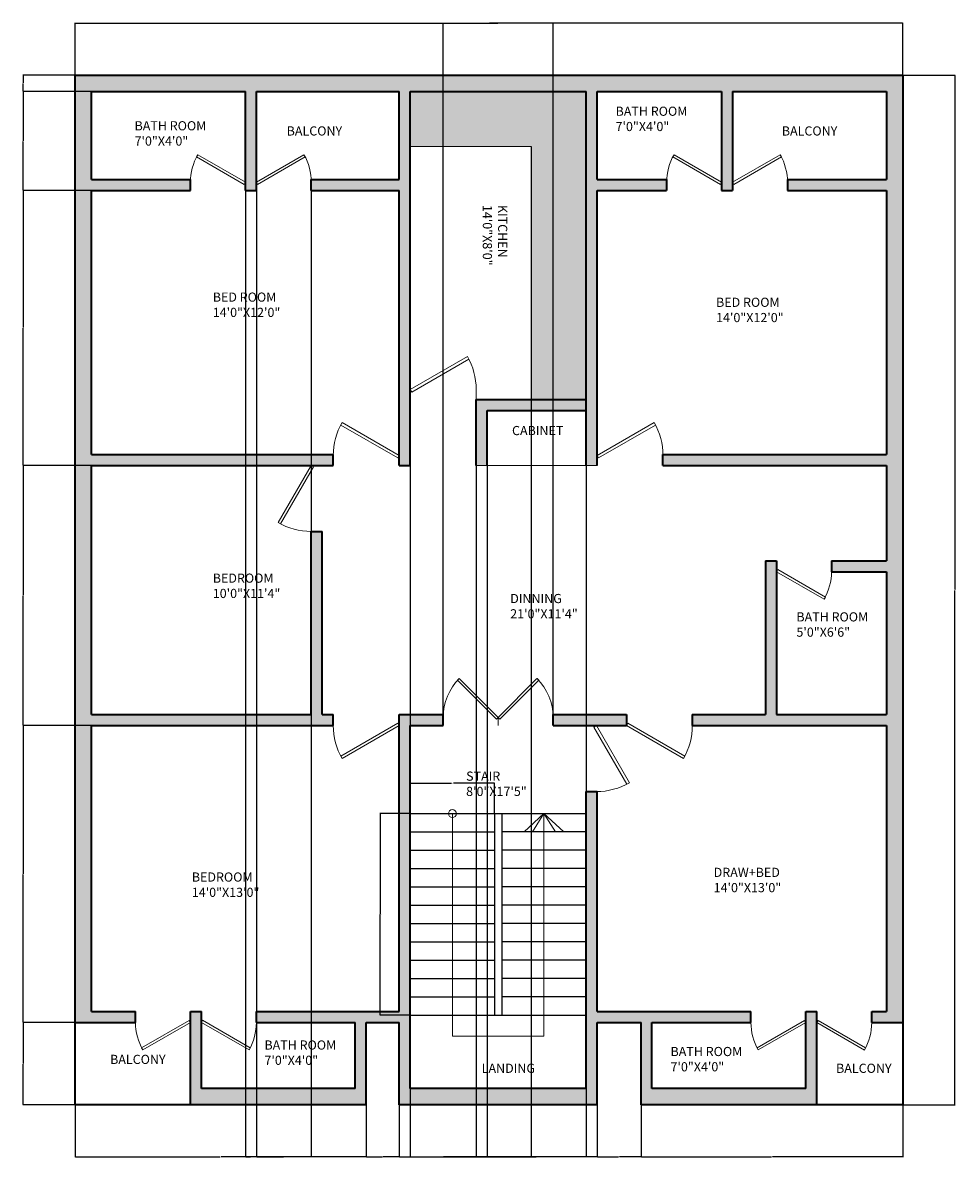
# Model space of a CAD drawing. Units: feet. Extents: x 3441 to 3951, y 1231 to 1850.
import ezdxf

# ---------------------------------------------------------------- set-up
doc = ezdxf.new("R2010")
doc.units = ezdxf.units.FT
for name, color, linetype, lineweight in [('A-ANNO-DIMS', 2, 'Continuous', 18), ('A-ANNO-SYMB', 130, 'Continuous', 13), ('A-AREA-IDEN', 170, 'Continuous', 18), ('A-FLOR-CASE', 7, 'Continuous', 18), ('A-FLOR-CASE-PATT', 8, 'Continuous', 13), ('A-WALL', 7, 'Continuous', 35), ('DOOR', 119, 'Continuous', 18), ('STAIR CASE', 130, 'Continuous', 25)]:
    doc.layers.add(name, color=color, linetype=linetype, lineweight=lineweight)
doc.layers.add('A-WALL-PATT', color=244, linetype='Continuous', lineweight=13, true_color=0x991b1e)
doc.styles.get("Standard").update_dxf_attribs({"font": 'arial.ttf'})
doc.dimstyles.get("Standard").update_dxf_attribs({"dimtxt": 0.18, "dimasz": 0.18, "dimexe": 0.18, "dimexo": 0.0625, "dimgap": 0.09, "dimtad": 0, "dimtih": 1, "dimtoh": 1, "dimdec": 4, "dimzin": 0, "dimdsep": 46, "dimtxsty": 'Standard', "dimcen": 0.09, "dimadec": 0, "dimazin": 0, "dimtfac": 1, "dimtdec": 4, "dimtofl": 0, "dimtmove": 0, "dimatfit": 3, "dimfxl": 1, "dimtolj": 1, "dimtzin": 0, "dimarcsym": 0})

# ---------------------------------------------------------------- blocks, each defined once
blk = doc.blocks.new('*U5')
for p, q in [((0, 0), (0, -6)), ((40, 0), (40, -6))]:
    blk.add_line(p, q)
blk.add_lwpolyline([(0, 0), (34.64, 20), (35.52, 18.48), (0.87, -1.52)], close=True)
blk.add_arc((0, 0), 40, 0, 30)
blk = doc.blocks.new('*U6')
for p, q in [((0, 0), (0, -6)), ((-40, 0), (-40, -6))]:
    blk.add_line(p, q)
blk.add_lwpolyline([(0, 0), (-34.64, 20), (-35.52, 18.48), (-0.88, -1.52)], close=True)
blk.add_arc((0, 0), 40, 150, 180)
blk = doc.blocks.new('*U4')
for p, q in [((0, 0), (0, -6)), ((-40, 0), (-40, -6))]:
    blk.add_line(p, q)
blk.add_lwpolyline([(0, 0), (-34.64, 20), (-35.52, 18.48), (-0.88, -1.52)], close=True)
blk.add_arc((0, 0), 40, 150, 180)
blk = doc.blocks.new('*U3')
for p, q in [((-40, 0), (-40, 6)), ((0, 0), (0, 6))]:
    blk.add_line(p, q)
blk.add_lwpolyline([(0, 0), (-34.64, -20), (-35.52, -18.48), (-0.87, 1.52)], close=True)
blk.add_arc((0, 0), 40, 180, 210)
blk = doc.blocks.new('*U2')
for p, q in [((0, 0), (0, 6)), ((40, 0), (40, 6))]:
    blk.add_line(p, q)
blk.add_lwpolyline([(0, 0), (34.64, -20), (35.52, -18.48), (0.87, 1.52)], close=True)
blk.add_arc((0, 0), 40, 330, 0)
blk = doc.blocks.new('*U7')
for p, q in [((0, 0), (0, 6)), ((40, 0), (40, 6))]:
    blk.add_line(p, q)
blk.add_lwpolyline([(0, 0), (34.64, -20), (35.52, -18.48), (0.87, 1.52)], close=True)
blk.add_arc((0, 0), 40, 330, 0)
blk = doc.blocks.new('*U9')
for p, q in [((-40, 0), (-40, 6)), ((0, 0), (0, 6))]:
    blk.add_line(p, q)
blk.add_lwpolyline([(0, 0), (-34.64, -20), (-35.52, -18.48), (-0.88, 1.52)], close=True)
blk.add_arc((0, 0), 40, 180, 210)
blk = doc.blocks.new('*U8')
for p, q in [((0, 0), (0, -6)), ((-40, 0), (-40, -6))]:
    blk.add_line(p, q)
blk.add_lwpolyline([(0, 0), (-34.64, 20), (-35.52, 18.48), (-0.88, -1.52)], close=True)
blk.add_arc((0, 0), 40, 150, 180)
blk = doc.blocks.new('*U10')
for p, q in [((0, 0), (0, -6)), ((40, 0), (40, -6))]:
    blk.add_line(p, q)
blk.add_lwpolyline([(0, 0), (28.28, 28.28), (29.52, 27.05), (1.24, -1.24)], close=True)
blk.add_arc((0, 0), 40, 0, 45)
blk = doc.blocks.new('STAIR-FLIGHT-46IN')
for p, q in [((46, 110), (46, 0)), ((0, 100), (46, 100)), ((0, 90), (46, 90)), ((0, 80), (46, 80)), ((0, 70), (46, 70)), ((0, 60), (46, 60)), ((0, 50), (46, 50)), ((0, 40), (46, 40)), ((0, 30), (46, 30)), ((0, 20), (46, 20)), ((0, 20), (46, 20)), ((0, 10), (46, 10))]:
    blk.add_line(p, q)
blk = doc.blocks.new('*D12')
at = {"layer": 'A-ANNO-DIMS', "color": 0, "lineweight": -2, "transparency": 16777216}
for p, q in [((3652.89, 1418.79), (3636.27, 1418.79)), ((3636.45, 1418.61), (3636.45, 1363.97)), ((3636.45, 1308.97), (3636.45, 1363.6)), ((3652.89, 1308.79), (3636.27, 1308.79))]:
    blk.add_line(p, q, dxfattribs=at)
at = {"layer": 'A-ANNO-DIMS', "color": 0, "transparency": 16777216}
for points in [[(3636.42, 1418.61), (3636.48, 1418.61), (3636.45, 1418.79)], [(3636.42, 1308.97), (3636.48, 1308.97), (3636.45, 1308.79)]]:
    blk.add_solid(points, dxfattribs=at)
at = {"layer": 'Defpoints', "color": 0, "transparency": 16777216}
for p in [(3636.45, 1418.79), (3652.95, 1418.79), (3652.95, 1308.79)]:
    blk.add_point(p, dxfattribs=at)
at = {"layer": 'A-ANNO-DIMS', "color": 0, "transparency": 16777216, "insert": (3636.45, 1363.79), "char_height": 0.18, "attachment_point": 5}
blk.add_mtext('\\A1;FLIGHT 110 TYP.', dxfattribs=at)
blk = doc.blocks.new('*D13')
at = {"layer": 'A-ANNO-DIMS', "color": 0, "lineweight": -2, "transparency": 16777216}
for p, q in [((3652.95, 1418.85), (3652.95, 1435.47)), ((3653.13, 1435.29), (3675.42, 1435.29)), ((3698.77, 1435.29), (3676.49, 1435.29)), ((3698.95, 1418.85), (3698.95, 1435.47))]:
    blk.add_line(p, q, dxfattribs=at)
at = {"layer": 'A-ANNO-DIMS', "color": 0, "transparency": 16777216}
for points in [[(3653.13, 1435.32), (3653.13, 1435.26), (3652.95, 1435.29)], [(3698.77, 1435.32), (3698.77, 1435.26), (3698.95, 1435.29)]]:
    blk.add_solid(points, dxfattribs=at)
at = {"layer": 'Defpoints', "color": 0, "transparency": 16777216}
for p in [(3698.95, 1435.29), (3652.95, 1418.79), (3698.95, 1418.79)]:
    blk.add_point(p, dxfattribs=at)
at = {"layer": 'A-ANNO-DIMS', "color": 0, "transparency": 16777216, "insert": (3675.95, 1435.29), "char_height": 0.18, "attachment_point": 5}
blk.add_mtext('\\A1;46 TYP.', dxfattribs=at)
blk = doc.blocks.new('*D14')
at = {"layer": 'A-ANNO-DIMS', "color": 0, "lineweight": -2, "transparency": 16777216}
for p, q in [((3469.95, 1821.85), (3469.95, 1850.37)), ((3470.13, 1850.19), (3695.66, 1850.19)), ((3921.77, 1850.19), (3696.25, 1850.19)), ((3921.95, 1821.85), (3921.95, 1850.37))]:
    blk.add_line(p, q, dxfattribs=at)
at = {"layer": 'A-ANNO-DIMS', "color": 0, "transparency": 16777216}
for points in [[(3470.13, 1850.22), (3470.13, 1850.16), (3469.95, 1850.19)], [(3921.77, 1850.22), (3921.77, 1850.16), (3921.95, 1850.19)]]:
    blk.add_solid(points, dxfattribs=at)
at = {"layer": 'Defpoints', "color": 0, "transparency": 16777216}
for p in [(3921.95, 1850.19), (3469.95, 1821.79), (3921.95, 1821.79)]:
    blk.add_point(p, dxfattribs=at)
at = {"layer": 'A-ANNO-DIMS', "color": 0, "transparency": 16777216, "insert": (3695.95, 1850.19), "char_height": 0.18, "attachment_point": 5}
blk.add_mtext('\\A1;452', dxfattribs=at)
blk = doc.blocks.new('*D15')
at = {"layer": 'A-ANNO-DIMS', "color": 0, "lineweight": -2, "transparency": 16777216}
for p, q in [((3922.02, 1821.79), (3950.53, 1821.79)), ((3950.35, 1821.61), (3950.35, 1540.97)), ((3950.35, 1259.97), (3950.35, 1540.6)), ((3922.02, 1259.79), (3950.53, 1259.79))]:
    blk.add_line(p, q, dxfattribs=at)
at = {"layer": 'A-ANNO-DIMS', "color": 0, "transparency": 16777216}
for points in [[(3950.32, 1821.61), (3950.38, 1821.61), (3950.35, 1821.79)], [(3950.32, 1259.97), (3950.38, 1259.97), (3950.35, 1259.79)]]:
    blk.add_solid(points, dxfattribs=at)
at = {"layer": 'Defpoints', "color": 0, "transparency": 16777216}
for p in [(3921.95, 1821.79), (3950.35, 1821.79), (3921.95, 1259.79)]:
    blk.add_point(p, dxfattribs=at)
at = {"layer": 'A-ANNO-DIMS', "color": 0, "transparency": 16777216, "insert": (3950.35, 1540.79), "char_height": 0.18, "attachment_point": 5}
blk.add_mtext('\\A1;562', dxfattribs=at)
blk = doc.blocks.new('*D16')
at = {"layer": 'A-ANNO-DIMS', "color": 0, "lineweight": -2, "transparency": 16777216}
for p, q in [((3469.95, 1259.72), (3469.95, 1231.21)), ((3628.95, 1259.72), (3628.95, 1231.21)), ((3470.13, 1231.39), (3549.17, 1231.39)), ((3628.77, 1231.39), (3549.73, 1231.39))]:
    blk.add_line(p, q, dxfattribs=at)
at = {"layer": 'A-ANNO-DIMS', "color": 0, "transparency": 16777216}
for points in [[(3470.13, 1231.42), (3470.13, 1231.36), (3469.95, 1231.39)], [(3628.77, 1231.42), (3628.77, 1231.36), (3628.95, 1231.39)]]:
    blk.add_solid(points, dxfattribs=at)
at = {"layer": 'Defpoints', "color": 0, "transparency": 16777216}
for p in [(3469.95, 1259.79), (3628.95, 1259.79), (3628.95, 1231.39)]:
    blk.add_point(p, dxfattribs=at)
at = {"layer": 'A-ANNO-DIMS', "color": 0, "transparency": 16777216, "insert": (3549.45, 1231.39), "char_height": 0.18, "attachment_point": 5}
blk.add_mtext('\\A1;159', dxfattribs=at)
blk = doc.blocks.new('*D17')
at = {"layer": 'A-ANNO-DIMS', "color": 0, "lineweight": -2, "transparency": 16777216}
for p, q in [((3628.95, 1259.72), (3628.95, 1231.21)), ((3646.95, 1259.72), (3646.95, 1231.21)), ((3629.13, 1231.39), (3637.74, 1231.39)), ((3646.77, 1231.39), (3638.16, 1231.39))]:
    blk.add_line(p, q, dxfattribs=at)
at = {"layer": 'A-ANNO-DIMS', "color": 0, "transparency": 16777216}
for points in [[(3629.13, 1231.42), (3629.13, 1231.36), (3628.95, 1231.39)], [(3646.77, 1231.42), (3646.77, 1231.36), (3646.95, 1231.39)]]:
    blk.add_solid(points, dxfattribs=at)
at = {"layer": 'Defpoints', "color": 0, "transparency": 16777216}
for p in [(3628.95, 1259.79), (3646.95, 1259.79), (3646.95, 1231.39)]:
    blk.add_point(p, dxfattribs=at)
at = {"layer": 'A-ANNO-DIMS', "color": 0, "transparency": 16777216, "insert": (3637.95, 1231.39), "char_height": 0.18, "attachment_point": 5}
blk.add_mtext('\\A1;18', dxfattribs=at)
blk = doc.blocks.new('*D18')
at = {"layer": 'A-ANNO-DIMS', "color": 0, "lineweight": -2, "transparency": 16777216}
for p, q in [((3646.95, 1259.72), (3646.95, 1231.21)), ((3754.95, 1259.72), (3754.95, 1231.21)), ((3647.13, 1231.39), (3700.67, 1231.39)), ((3754.77, 1231.39), (3701.23, 1231.39))]:
    blk.add_line(p, q, dxfattribs=at)
at = {"layer": 'A-ANNO-DIMS', "color": 0, "transparency": 16777216}
for points in [[(3647.13, 1231.42), (3647.13, 1231.36), (3646.95, 1231.39)], [(3754.77, 1231.42), (3754.77, 1231.36), (3754.95, 1231.39)]]:
    blk.add_solid(points, dxfattribs=at)
at = {"layer": 'Defpoints', "color": 0, "transparency": 16777216}
for p in [(3646.95, 1259.79), (3754.95, 1259.79), (3754.95, 1231.39)]:
    blk.add_point(p, dxfattribs=at)
at = {"layer": 'A-ANNO-DIMS', "color": 0, "transparency": 16777216, "insert": (3700.95, 1231.39), "char_height": 0.18, "attachment_point": 5}
blk.add_mtext('\\A1;108', dxfattribs=at)
blk = doc.blocks.new('*D19')
at = {"layer": 'A-ANNO-DIMS', "color": 0, "lineweight": -2, "transparency": 16777216}
for p, q in [((3754.95, 1259.72), (3754.95, 1231.21)), ((3778.95, 1259.72), (3778.95, 1231.21)), ((3755.13, 1231.39), (3766.73, 1231.39)), ((3778.77, 1231.39), (3767.17, 1231.39))]:
    blk.add_line(p, q, dxfattribs=at)
at = {"layer": 'A-ANNO-DIMS', "color": 0, "transparency": 16777216}
for points in [[(3755.13, 1231.42), (3755.13, 1231.36), (3754.95, 1231.39)], [(3778.77, 1231.42), (3778.77, 1231.36), (3778.95, 1231.39)]]:
    blk.add_solid(points, dxfattribs=at)
at = {"layer": 'Defpoints', "color": 0, "transparency": 16777216}
for p in [(3754.95, 1259.79), (3778.95, 1259.79), (3778.95, 1231.39)]:
    blk.add_point(p, dxfattribs=at)
at = {"layer": 'A-ANNO-DIMS', "color": 0, "transparency": 16777216, "insert": (3766.95, 1231.39), "char_height": 0.18, "attachment_point": 5}
blk.add_mtext('\\A1;24', dxfattribs=at)
blk = doc.blocks.new('*D20')
at = {"layer": 'A-ANNO-DIMS', "color": 0, "lineweight": -2, "transparency": 16777216}
for p, q in [((3778.95, 1259.72), (3778.95, 1231.21)), ((3921.95, 1259.72), (3921.95, 1231.21)), ((3779.13, 1231.39), (3850.17, 1231.39)), ((3921.77, 1231.39), (3850.73, 1231.39))]:
    blk.add_line(p, q, dxfattribs=at)
at = {"layer": 'A-ANNO-DIMS', "color": 0, "transparency": 16777216}
for points in [[(3779.13, 1231.42), (3779.13, 1231.36), (3778.95, 1231.39)], [(3921.77, 1231.42), (3921.77, 1231.36), (3921.95, 1231.39)]]:
    blk.add_solid(points, dxfattribs=at)
at = {"layer": 'Defpoints', "color": 0, "transparency": 16777216}
for p in [(3778.95, 1259.79), (3921.95, 1259.79), (3921.95, 1231.39)]:
    blk.add_point(p, dxfattribs=at)
at = {"layer": 'A-ANNO-DIMS', "color": 0, "transparency": 16777216, "insert": (3850.45, 1231.39), "char_height": 0.18, "attachment_point": 5}
blk.add_mtext('\\A1;143', dxfattribs=at)
blk = doc.blocks.new('*D21')
at = {"layer": 'A-ANNO-DIMS', "color": 0, "lineweight": -2, "transparency": 16777216}
for p, q in [((3469.89, 1304.79), (3441.37, 1304.79)), ((3441.55, 1304.61), (3441.55, 1282.47)), ((3441.55, 1259.97), (3441.55, 1282.1)), ((3469.89, 1259.79), (3441.37, 1259.79))]:
    blk.add_line(p, q, dxfattribs=at)
at = {"layer": 'A-ANNO-DIMS', "color": 0, "transparency": 16777216}
for points in [[(3441.52, 1304.61), (3441.58, 1304.61), (3441.55, 1304.79)], [(3441.52, 1259.97), (3441.58, 1259.97), (3441.55, 1259.79)]]:
    blk.add_solid(points, dxfattribs=at)
at = {"layer": 'Defpoints', "color": 0, "transparency": 16777216}
for p in [(3441.55, 1304.79), (3469.95, 1304.79), (3469.95, 1259.79)]:
    blk.add_point(p, dxfattribs=at)
at = {"layer": 'A-ANNO-DIMS', "color": 0, "transparency": 16777216, "insert": (3441.55, 1282.29), "char_height": 0.18, "attachment_point": 5}
blk.add_mtext('\\A1;45', dxfattribs=at)
blk = doc.blocks.new('*D22')
at = {"layer": 'A-ANNO-DIMS', "color": 0, "lineweight": -2, "transparency": 16777216}
for p, q in [((3478.89, 1466.79), (3441.37, 1466.79)), ((3441.55, 1466.61), (3441.55, 1385.97)), ((3441.55, 1304.97), (3441.55, 1385.6)), ((3469.89, 1304.79), (3441.37, 1304.79))]:
    blk.add_line(p, q, dxfattribs=at)
at = {"layer": 'A-ANNO-DIMS', "color": 0, "transparency": 16777216}
for points in [[(3441.52, 1466.61), (3441.58, 1466.61), (3441.55, 1466.79)], [(3441.52, 1304.97), (3441.58, 1304.97), (3441.55, 1304.79)]]:
    blk.add_solid(points, dxfattribs=at)
at = {"layer": 'Defpoints', "color": 0, "transparency": 16777216}
for p in [(3441.55, 1466.79), (3478.95, 1466.79), (3469.95, 1304.79)]:
    blk.add_point(p, dxfattribs=at)
at = {"layer": 'A-ANNO-DIMS', "color": 0, "transparency": 16777216, "insert": (3441.55, 1385.79), "char_height": 0.18, "attachment_point": 5}
blk.add_mtext('\\A1;162', dxfattribs=at)
blk = doc.blocks.new('*D23')
at = {"layer": 'A-ANNO-DIMS', "color": 0, "lineweight": -2, "transparency": 16777216}
for p, q in [((3478.89, 1608.79), (3441.37, 1608.79)), ((3441.55, 1608.61), (3441.55, 1537.97)), ((3441.55, 1466.97), (3441.55, 1537.61)), ((3478.89, 1466.79), (3441.37, 1466.79))]:
    blk.add_line(p, q, dxfattribs=at)
at = {"layer": 'A-ANNO-DIMS', "color": 0, "transparency": 16777216}
for points in [[(3441.52, 1608.61), (3441.58, 1608.61), (3441.55, 1608.79)], [(3441.52, 1466.97), (3441.58, 1466.97), (3441.55, 1466.79)]]:
    blk.add_solid(points, dxfattribs=at)
at = {"layer": 'Defpoints', "color": 0, "transparency": 16777216}
for p in [(3441.55, 1608.79), (3478.95, 1608.79), (3478.95, 1466.79)]:
    blk.add_point(p, dxfattribs=at)
at = {"layer": 'A-ANNO-DIMS', "color": 0, "transparency": 16777216, "insert": (3441.55, 1537.79), "char_height": 0.18, "attachment_point": 5}
blk.add_mtext('\\A1;142', dxfattribs=at)
blk = doc.blocks.new('*D24')
at = {"layer": 'A-ANNO-DIMS', "color": 0, "lineweight": -2, "transparency": 16777216}
for p, q in [((3478.89, 1758.79), (3441.37, 1758.79)), ((3441.55, 1758.61), (3441.55, 1683.97)), ((3441.55, 1608.97), (3441.55, 1683.6)), ((3478.89, 1608.79), (3441.37, 1608.79))]:
    blk.add_line(p, q, dxfattribs=at)
at = {"layer": 'A-ANNO-DIMS', "color": 0, "transparency": 16777216}
for points in [[(3441.52, 1758.61), (3441.58, 1758.61), (3441.55, 1758.79)], [(3441.52, 1608.97), (3441.58, 1608.97), (3441.55, 1608.79)]]:
    blk.add_solid(points, dxfattribs=at)
at = {"layer": 'Defpoints', "color": 0, "transparency": 16777216}
for p in [(3441.55, 1758.79), (3478.95, 1758.79), (3478.95, 1608.79)]:
    blk.add_point(p, dxfattribs=at)
at = {"layer": 'A-ANNO-DIMS', "color": 0, "transparency": 16777216, "insert": (3441.55, 1683.79), "char_height": 0.18, "attachment_point": 5}
blk.add_mtext('\\A1;150', dxfattribs=at)
blk = doc.blocks.new('*D25')
at = {"layer": 'A-ANNO-DIMS', "color": 0, "lineweight": -2, "transparency": 16777216}
for p, q in [((3478.89, 1812.79), (3441.37, 1812.79)), ((3441.55, 1812.61), (3441.55, 1785.97)), ((3441.55, 1758.97), (3441.55, 1785.6)), ((3478.89, 1758.79), (3441.37, 1758.79))]:
    blk.add_line(p, q, dxfattribs=at)
at = {"layer": 'A-ANNO-DIMS', "color": 0, "transparency": 16777216}
for points in [[(3441.52, 1812.61), (3441.58, 1812.61), (3441.55, 1812.79)], [(3441.52, 1758.97), (3441.58, 1758.97), (3441.55, 1758.79)]]:
    blk.add_solid(points, dxfattribs=at)
at = {"layer": 'Defpoints', "color": 0, "transparency": 16777216}
for p in [(3441.55, 1812.79), (3478.95, 1812.79), (3478.95, 1758.79)]:
    blk.add_point(p, dxfattribs=at)
at = {"layer": 'A-ANNO-DIMS', "color": 0, "transparency": 16777216, "insert": (3441.55, 1785.79), "char_height": 0.18, "attachment_point": 5}
blk.add_mtext('\\A1;54', dxfattribs=at)
blk = doc.blocks.new('*D26')
at = {"layer": 'A-ANNO-DIMS', "color": 0, "lineweight": -2, "transparency": 16777216}
for p, q in [((3469.89, 1821.79), (3441.37, 1821.79)), ((3441.55, 1821.61), (3441.55, 1817.47)), ((3441.55, 1812.97), (3441.55, 1817.1)), ((3478.89, 1812.79), (3441.37, 1812.79))]:
    blk.add_line(p, q, dxfattribs=at)
at = {"layer": 'A-ANNO-DIMS', "color": 0, "transparency": 16777216}
for points in [[(3441.52, 1821.61), (3441.58, 1821.61), (3441.55, 1821.79)], [(3441.52, 1812.97), (3441.58, 1812.97), (3441.55, 1812.79)]]:
    blk.add_solid(points, dxfattribs=at)
at = {"layer": 'Defpoints', "color": 0, "transparency": 16777216}
for p in [(3441.55, 1821.79), (3469.95, 1821.79), (3478.95, 1812.79)]:
    blk.add_point(p, dxfattribs=at)
at = {"layer": 'A-ANNO-DIMS', "color": 0, "transparency": 16777216, "insert": (3441.55, 1817.29), "char_height": 0.18, "attachment_point": 5}
blk.add_mtext('\\A1;9', dxfattribs=at)
blk = doc.blocks.new('*D27')
at = {"layer": 'A-ANNO-DIMS', "color": 0, "lineweight": -2, "transparency": 16777216}
for p, q in [((3670.95, 1472.85), (3670.95, 1850.37)), ((3671.13, 1850.19), (3700.74, 1850.19)), ((3730.77, 1850.19), (3701.17, 1850.19)), ((3730.95, 1472.85), (3730.95, 1850.37))]:
    blk.add_line(p, q, dxfattribs=at)
at = {"layer": 'A-ANNO-DIMS', "color": 0, "transparency": 16777216}
for points in [[(3671.13, 1850.22), (3671.13, 1850.16), (3670.95, 1850.19)], [(3730.77, 1850.22), (3730.77, 1850.16), (3730.95, 1850.19)]]:
    blk.add_solid(points, dxfattribs=at)
at = {"layer": 'Defpoints', "color": 0, "transparency": 16777216}
for p in [(3730.95, 1850.19), (3670.95, 1472.79), (3730.95, 1472.79)]:
    blk.add_point(p, dxfattribs=at)
at = {"layer": 'A-ANNO-DIMS', "color": 0, "transparency": 16777216, "insert": (3700.95, 1850.19), "char_height": 0.18, "attachment_point": 5}
blk.add_mtext('\\A1;60', dxfattribs=at)
blk = doc.blocks.new('*D28')
at = {"layer": 'A-ANNO-DIMS', "color": 0, "lineweight": -2, "transparency": 16777216}
for p, q in [((3652.95, 1644.72), (3652.95, 1231.21)), ((3688.95, 1644.72), (3688.95, 1231.21)), ((3653.13, 1231.39), (3670.74, 1231.39)), ((3688.77, 1231.39), (3671.17, 1231.39))]:
    blk.add_line(p, q, dxfattribs=at)
at = {"layer": 'A-ANNO-DIMS', "color": 0, "transparency": 16777216}
for points in [[(3653.13, 1231.42), (3653.13, 1231.36), (3652.95, 1231.39)], [(3688.77, 1231.42), (3688.77, 1231.36), (3688.95, 1231.39)]]:
    blk.add_solid(points, dxfattribs=at)
at = {"layer": 'Defpoints', "color": 0, "transparency": 16777216}
for p in [(3652.95, 1644.79), (3688.95, 1644.79), (3688.95, 1231.39)]:
    blk.add_point(p, dxfattribs=at)
at = {"layer": 'A-ANNO-DIMS', "color": 0, "transparency": 16777216, "insert": (3670.95, 1231.39), "char_height": 0.18, "attachment_point": 5}
blk.add_mtext('\\A1;36', dxfattribs=at)
blk = doc.blocks.new('*D29')
at = {"layer": 'A-ANNO-DIMS', "color": 0, "lineweight": -2, "transparency": 16777216}
for p, q in [((3568.95, 1758.72), (3568.95, 1231.21)), ((3598.95, 1758.72), (3598.95, 1231.21)), ((3569.13, 1231.39), (3583.74, 1231.39)), ((3598.77, 1231.39), (3584.17, 1231.39))]:
    blk.add_line(p, q, dxfattribs=at)
at = {"layer": 'A-ANNO-DIMS', "color": 0, "transparency": 16777216}
for points in [[(3569.13, 1231.42), (3569.13, 1231.36), (3568.95, 1231.39)], [(3598.77, 1231.42), (3598.77, 1231.36), (3598.95, 1231.39)]]:
    blk.add_solid(points, dxfattribs=at)
at = {"layer": 'Defpoints', "color": 0, "transparency": 16777216}
for p in [(3568.95, 1758.79), (3598.95, 1758.79), (3598.95, 1231.39)]:
    blk.add_point(p, dxfattribs=at)
at = {"layer": 'A-ANNO-DIMS', "color": 0, "transparency": 16777216, "insert": (3583.95, 1231.39), "char_height": 0.18, "attachment_point": 5}
blk.add_mtext('\\A1;30', dxfattribs=at)
blk = doc.blocks.new('*D30')
at = {"layer": 'A-ANNO-DIMS', "color": 0, "lineweight": -2, "transparency": 16777216}
for p, q in [((3694.95, 1608.72), (3694.95, 1231.21)), ((3748.95, 1608.72), (3748.95, 1231.21)), ((3695.13, 1231.39), (3721.74, 1231.39)), ((3748.77, 1231.39), (3722.17, 1231.39))]:
    blk.add_line(p, q, dxfattribs=at)
at = {"layer": 'A-ANNO-DIMS', "color": 0, "transparency": 16777216}
for points in [[(3695.13, 1231.42), (3695.13, 1231.36), (3694.95, 1231.39)], [(3748.77, 1231.42), (3748.77, 1231.36), (3748.95, 1231.39)]]:
    blk.add_solid(points, dxfattribs=at)
at = {"layer": 'Defpoints', "color": 0, "transparency": 16777216}
for p in [(3694.95, 1608.79), (3748.95, 1608.79), (3748.95, 1231.39)]:
    blk.add_point(p, dxfattribs=at)
at = {"layer": 'A-ANNO-DIMS', "color": 0, "transparency": 16777216, "insert": (3721.95, 1231.39), "char_height": 0.18, "attachment_point": 5}
blk.add_mtext('\\A1;54', dxfattribs=at)
blk = doc.blocks.new('*D31')
at = {"layer": 'A-ANNO-DIMS', "color": 0, "lineweight": -2, "transparency": 16777216}
for p, q in [((3562.95, 1758.72), (3562.95, 1231.21)), ((3568.95, 1758.72), (3568.95, 1231.21)), ((3563.13, 1231.39), (3565.8, 1231.39)), ((3568.77, 1231.39), (3566.1, 1231.39))]:
    blk.add_line(p, q, dxfattribs=at)
at = {"layer": 'A-ANNO-DIMS', "color": 0, "transparency": 16777216}
for points in [[(3563.13, 1231.42), (3563.13, 1231.36), (3562.95, 1231.39)], [(3568.77, 1231.42), (3568.77, 1231.36), (3568.95, 1231.39)]]:
    blk.add_solid(points, dxfattribs=at)
at = {"layer": 'Defpoints', "color": 0, "transparency": 16777216}
for p in [(3562.95, 1758.79), (3568.95, 1758.79), (3568.95, 1231.39)]:
    blk.add_point(p, dxfattribs=at)
at = {"layer": 'A-ANNO-DIMS', "color": 0, "transparency": 16777216, "insert": (3565.95, 1231.39), "char_height": 0.18, "attachment_point": 5}
blk.add_mtext('\\A1;6', dxfattribs=at)
blk = doc.blocks.new('*D32')
at = {"layer": 'A-ANNO-DIMS', "color": 0, "lineweight": -2, "transparency": 16777216}
for p, q in [((3652.95, 1782.72), (3652.95, 1231.21)), ((3718.95, 1782.72), (3718.95, 1231.21)), ((3653.13, 1231.39), (3685.73, 1231.39)), ((3718.77, 1231.39), (3686.17, 1231.39))]:
    blk.add_line(p, q, dxfattribs=at)
at = {"layer": 'A-ANNO-DIMS', "color": 0, "transparency": 16777216}
for points in [[(3653.13, 1231.42), (3653.13, 1231.36), (3652.95, 1231.39)], [(3718.77, 1231.42), (3718.77, 1231.36), (3718.95, 1231.39)]]:
    blk.add_solid(points, dxfattribs=at)
at = {"layer": 'Defpoints', "color": 0, "transparency": 16777216}
for p in [(3652.95, 1782.79), (3718.95, 1782.79), (3718.95, 1231.39)]:
    blk.add_point(p, dxfattribs=at)
at = {"layer": 'A-ANNO-DIMS', "color": 0, "transparency": 16777216, "insert": (3685.95, 1231.39), "char_height": 0.18, "attachment_point": 5}
blk.add_mtext('\\A1;66', dxfattribs=at)

msp = doc.modelspace()

# ---------------------------------------------------------------- hatches: boundary and pattern name
at = {"layer": 'A-FLOR-CASE-PATT'}
h = msp.add_hatch(color=256, dxfattribs=at)
h.dxf.hatch_style = 1
h.paths.add_polyline_path([(3748.95, 1812.79), (3652.95, 1812.79), (3652.95, 1782.79), (3718.95, 1782.79), (3718.95, 1644.79), (3748.95, 1644.79)])
at = {"layer": 'A-WALL-PATT'}
h = msp.add_hatch(color=256, dxfattribs=at)
h.dxf.hatch_style = 1
h.paths.add_polyline_path([(3694.95, 1638.79), (3748.95, 1638.79), (3748.95, 1644.79), (3688.95, 1644.79), (3688.95, 1608.79), (3694.95, 1608.79)], flags=17)
h.paths.add_polyline_path([(3754.95, 1758.79), (3792.95, 1758.79), (3792.95, 1764.79), (3754.95, 1764.79), (3754.95, 1812.79), (3822.95, 1812.79), (3822.95, 1758.79), (3828.95, 1758.79), (3828.95, 1812.79), (3912.95, 1812.79), (3912.95, 1764.79), (3858.95, 1764.79), (3858.95, 1758.79), (3912.95, 1758.79), (3912.95, 1614.79), (3790.95, 1614.79), (3790.95, 1608.79), (3912.95, 1608.79), (3912.95, 1556.79), (3882.95, 1556.79), (3882.95, 1550.79), (3912.95, 1550.79), (3912.95, 1472.79), (3852.95, 1472.79), (3852.95, 1556.79), (3846.95, 1556.79), (3846.95, 1466.79), (3912.95, 1466.79), (3912.95, 1310.79), (3904.95, 1310.79), (3904.95, 1304.79), (3921.95, 1304.79), (3921.95, 1821.79), (3469.95, 1821.79), (3469.95, 1304.79), (3502.95, 1304.79), (3502.95, 1310.79), (3478.95, 1310.79), (3478.95, 1466.79), (3610.95, 1466.79), (3610.95, 1472.79), (3604.95, 1472.79), (3604.95, 1572.79), (3598.95, 1572.79), (3598.95, 1472.79), (3478.95, 1472.79), (3478.95, 1608.79), (3610.95, 1608.79), (3610.95, 1614.79), (3478.95, 1614.79), (3478.95, 1758.79), (3532.95, 1758.79), (3532.95, 1764.79), (3478.95, 1764.79), (3478.95, 1812.79), (3562.95, 1812.79), (3562.95, 1758.79), (3568.95, 1758.79), (3568.95, 1812.79), (3646.95, 1812.79), (3646.95, 1764.79), (3598.95, 1764.79), (3598.95, 1758.79), (3646.95, 1758.79), (3646.95, 1608.79), (3652.95, 1608.79), (3652.95, 1812.79), (3748.95, 1812.79), (3748.95, 1608.79), (3754.95, 1608.79)])
h.paths.add_polyline_path([(3538.95, 1310.79), (3532.95, 1310.79), (3532.95, 1259.79), (3628.95, 1259.79), (3628.95, 1304.79), (3646.95, 1304.79), (3646.95, 1268.79), (3646.95, 1259.79), (3652.95, 1259.79), (3652.95, 1268.79), (3652.95, 1466.79), (3670.95, 1466.79), (3670.95, 1472.79), (3646.95, 1472.79), (3646.95, 1310.79), (3568.95, 1310.79), (3568.95, 1304.79), (3622.95, 1304.79), (3622.95, 1268.79), (3538.95, 1268.79)])
h.paths.add_polyline_path([(3754.95, 1304.79), (3778.95, 1304.79), (3778.95, 1259.79), (3874.95, 1259.79), (3874.95, 1310.79), (3868.95, 1310.79), (3868.95, 1268.79), (3784.95, 1268.79), (3784.95, 1304.79), (3838.95, 1304.79), (3838.95, 1310.79), (3754.95, 1310.79), (3754.95, 1430.79), (3748.95, 1430.79), (3748.95, 1268.79), (3748.95, 1259.79), (3754.95, 1259.79), (3754.95, 1268.79)])
h.paths.add_polyline_path([(3748.95, 1268.79), (3652.95, 1268.79), (3652.95, 1259.79), (3748.95, 1259.79)])
h = msp.add_hatch(color=256, dxfattribs=at)
h.dxf.hatch_style = 1
h.paths.add_polyline_path([(3770.95, 1472.19), (3770.95, 1472.79), (3730.95, 1472.79), (3730.95, 1466.79), (3754.95, 1466.79), (3770.95, 1466.79)])
h.paths.add_polyline_path([(3846.95, 1472.79), (3806.95, 1472.79), (3806.95, 1466.79), (3846.95, 1466.79)])

# ---------------------------------------------------------------- linework, layer by layer
at = {"layer": 'A-ANNO-SYMB'}
for p, q in [((3675.95, 1408.79), (3675.95, 1418.79)), ((3725.95, 1418.79), (3715.18, 1408.79)), ((3725.95, 1418.79), (3719.65, 1408.79)), ((3725.95, 1297.39), (3725.95, 1418.79)), ((3725.95, 1418.79), (3732.26, 1408.79)), ((3725.95, 1418.79), (3736.73, 1408.79)), ((3675.95, 1408.79), (3675.95, 1297.39)), ((3675.95, 1297.39), (3725.95, 1297.39))]:
    msp.add_line(p, q, dxfattribs=at)
msp.add_circle((3675.95, 1418.79), 2.16, dxfattribs=at)
at = {"layer": 'A-FLOR-CASE'}
for p, q in [((3652.95, 1782.79), (3718.95, 1782.79)), ((3718.95, 1644.79), (3718.95, 1782.79)), ((3688.95, 1608.79), (3754.95, 1608.79))]:
    msp.add_line(p, q, dxfattribs=at)
at = {"layer": 'A-WALL'}
for p, q in [((3469.95, 1821.79), (3921.95, 1821.79)), ((3469.95, 1259.79), (3469.95, 1821.79)), ((3921.95, 1821.79), (3921.95, 1259.79)), ((3478.95, 1812.79), (3562.95, 1812.79)), ((3478.95, 1764.79), (3478.95, 1812.79)), ((3562.95, 1758.79), (3562.95, 1812.79)), ((3568.95, 1758.79), (3568.95, 1812.79)), ((3568.95, 1812.79), (3646.95, 1812.79)), ((3646.95, 1764.79), (3646.95, 1812.79)), ((3652.95, 1608.79), (3652.95, 1812.79)), ((3652.95, 1812.79), (3748.95, 1812.79)), ((3748.95, 1608.79), (3748.95, 1812.79)), ((3754.95, 1764.79), (3754.95, 1812.79)), ((3754.95, 1812.79), (3822.95, 1812.79)), ((3822.95, 1812.79), (3822.95, 1758.79)), ((3828.95, 1812.79), (3828.95, 1758.79)), ((3828.95, 1812.79), (3912.95, 1812.79)), ((3912.95, 1812.79), (3912.95, 1764.79)), ((3478.95, 1764.79), (3532.95, 1764.79)), ((3532.95, 1758.79), (3532.95, 1764.79)), ((3598.95, 1764.79), (3646.95, 1764.79)), ((3598.95, 1758.79), (3598.95, 1764.79)), ((3754.95, 1764.79), (3792.95, 1764.79)), ((3792.95, 1764.79), (3792.95, 1758.79)), ((3858.95, 1764.79), (3912.95, 1764.79)), ((3858.95, 1764.79), (3858.95, 1758.79)), ((3478.95, 1758.79), (3532.95, 1758.79)), ((3478.95, 1614.79), (3478.95, 1758.79)), ((3562.95, 1758.79), (3568.95, 1758.79)), ((3598.95, 1758.79), (3646.95, 1758.79)), ((3646.95, 1608.79), (3646.95, 1758.79)), ((3652.95, 1614.79), (3652.95, 1758.79)), ((3748.95, 1614.79), (3748.95, 1758.79)), ((3754.95, 1608.79), (3754.95, 1758.79)), ((3754.95, 1758.79), (3792.95, 1758.79)), ((3822.95, 1758.79), (3828.95, 1758.79)), ((3858.95, 1758.79), (3912.95, 1758.79)), ((3912.95, 1758.79), (3912.95, 1614.79)), ((3688.95, 1644.79), (3748.95, 1644.79)), ((3688.95, 1608.79), (3688.95, 1644.79)), ((3694.95, 1638.79), (3748.95, 1638.79)), ((3694.95, 1608.79), (3694.95, 1638.79)), ((3478.95, 1614.79), (3610.95, 1614.79)), ((3610.95, 1608.79), (3610.95, 1614.79)), ((3790.95, 1614.79), (3912.95, 1614.79)), ((3790.95, 1608.79), (3790.95, 1614.79)), ((3478.95, 1608.79), (3610.95, 1608.79)), ((3478.95, 1472.79), (3478.95, 1608.79)), ((3646.95, 1608.79), (3652.95, 1608.79)), ((3790.95, 1608.79), (3912.95, 1608.79)), ((3912.95, 1608.79), (3912.95, 1556.79)), ((3598.95, 1472.79), (3598.95, 1572.79)), ((3598.95, 1572.79), (3604.95, 1572.79)), ((3604.95, 1472.79), (3604.95, 1572.79)), ((3846.95, 1556.79), (3846.95, 1472.79)), ((3846.95, 1556.79), (3852.95, 1556.79)), ((3852.95, 1556.79), (3852.95, 1472.79)), ((3882.95, 1556.79), (3882.95, 1550.79)), ((3882.95, 1556.79), (3912.95, 1556.79)), ((3882.95, 1550.79), (3912.95, 1550.79)), ((3912.95, 1550.79), (3912.95, 1472.79)), ((3478.95, 1472.79), (3598.95, 1472.79)), ((3604.95, 1472.79), (3610.95, 1472.79)), ((3610.95, 1466.79), (3610.95, 1472.79)), ((3646.95, 1310.79), (3646.95, 1472.79)), ((3646.95, 1472.79), (3670.95, 1472.79)), ((3670.95, 1466.79), (3670.95, 1472.79)), ((3730.95, 1466.79), (3730.95, 1472.79)), ((3730.95, 1472.79), (3770.95, 1472.79)), ((3770.95, 1472.79), (3770.95, 1466.79)), ((3806.95, 1472.79), (3806.95, 1466.79)), ((3806.95, 1472.79), (3846.95, 1472.79)), ((3852.95, 1472.79), (3912.95, 1472.79)), ((3478.95, 1466.79), (3610.95, 1466.79)), ((3478.95, 1310.79), (3478.95, 1466.79)), ((3652.95, 1268.79), (3652.95, 1466.79)), ((3652.95, 1466.79), (3670.95, 1466.79)), ((3730.95, 1466.79), (3754.95, 1466.79)), ((3754.95, 1466.79), (3770.95, 1466.79)), ((3754.95, 1466.79), (3770.95, 1466.79)), ((3806.95, 1466.79), (3912.95, 1466.79)), ((3912.95, 1466.79), (3912.95, 1310.79)), ((3748.95, 1268.79), (3748.95, 1430.79)), ((3748.95, 1430.79), (3754.95, 1430.79)), ((3754.95, 1310.79), (3754.95, 1430.79)), ((3478.95, 1310.79), (3502.95, 1310.79)), ((3502.95, 1304.79), (3502.95, 1310.79)), ((3532.95, 1259.79), (3532.95, 1310.79)), ((3532.95, 1310.79), (3538.95, 1310.79)), ((3538.95, 1268.79), (3538.95, 1310.79)), ((3568.95, 1304.79), (3568.95, 1310.79)), ((3568.95, 1310.79), (3646.95, 1310.79)), ((3754.95, 1310.79), (3838.95, 1310.79)), ((3754.95, 1310.79), (3838.95, 1310.79)), ((3838.95, 1304.79), (3838.95, 1310.79)), ((3868.95, 1268.79), (3868.95, 1310.79)), ((3868.95, 1310.79), (3874.95, 1310.79)), ((3868.95, 1310.79), (3874.95, 1310.79)), ((3874.95, 1259.79), (3874.95, 1310.79)), ((3904.95, 1310.79), (3912.95, 1310.79)), ((3904.95, 1310.79), (3912.95, 1310.79)), ((3904.95, 1304.79), (3904.95, 1310.79)), ((3469.95, 1304.79), (3502.95, 1304.79)), ((3568.95, 1304.79), (3622.95, 1304.79)), ((3622.95, 1268.79), (3622.95, 1304.79)), ((3628.95, 1259.79), (3628.95, 1304.79)), ((3628.95, 1304.79), (3646.95, 1304.79)), ((3646.95, 1268.79), (3646.95, 1304.79)), ((3754.95, 1268.79), (3754.95, 1304.79)), ((3754.95, 1304.79), (3778.95, 1304.79)), ((3778.95, 1259.79), (3778.95, 1304.79)), ((3784.95, 1268.79), (3784.95, 1304.79)), ((3784.95, 1304.79), (3838.95, 1304.79)), ((3904.95, 1304.79), (3921.95, 1304.79)), ((3622.95, 1268.79), (3538.95, 1268.79)), ((3646.95, 1259.79), (3646.95, 1268.79)), ((3748.95, 1268.79), (3652.95, 1268.79)), ((3754.95, 1259.79), (3754.95, 1268.79)), ((3868.95, 1268.79), (3784.95, 1268.79)), ((3628.95, 1259.79), (3469.95, 1259.79)), ((3754.95, 1259.79), (3646.95, 1259.79)), ((3921.95, 1259.79), (3778.95, 1259.79))]:
    msp.add_line(p, q, dxfattribs=at)
at = {"layer": 'STAIR CASE'}
for p, q in [((3652.95, 1418.79), (3748.95, 1418.79)), ((3652.95, 1308.79), (3748.95, 1308.79))]:
    msp.add_line(p, q, dxfattribs=at)

# ---------------------------------------------------------------- block references
at = {"layer": 'DOOR'}
for name, p, xscale, yscale, zscale in [('*U4', (3562.95, 1763.29), 0.7499999999999659, 0.7499999999999659, 0.7499999999999659), ('*U5', (3568.95, 1763.29), 0.7499999999999659, 0.7499999999999659, 0.7499999999999659), ('*U6', (3822.95, 1763.29), 0.7499999999999659, 0.7499999999999659, 0.7499999999999659), ('*U5', (3828.95, 1763.29), 0.7499999999999659, 0.7499999999999659, 0.7499999999999659), ('*U8', (3652.95, 1650.19), -0.9, 0.9, 0.9), ('*U4', (3646.95, 1614.19), 0.9, 0.9, 0.9), ('*U5', (3754.95, 1614.19), 0.9, 0.9, 0.9), ('*U7', (3852.95, 1550.79), 0.7499999999999659, 0.7499999999999659, 0.7499999999999659), ('*U10', (3700.95, 1471.29), -0.7500000000000683, 0.7500000000000683, 0.7500000000000683), ('*U10', (3700.95, 1471.29), 0.7500000000000683, 0.7500000000000683, 0.7500000000000683), ('*U9', (3646.95, 1466.79), 0.9, 0.9, 0.9), ('*U2', (3770.95, 1466.79), 0.9, 0.9, 0.9), ('*U3', (3532.95, 1304.79), 0.7499999999999659, 0.7499999999999659, 0.7499999999999659), ('*U2', (3538.95, 1304.82), 0.7499999999999659, 0.7499999999999659, 0.7499999999999659), ('*U3', (3868.95, 1304.79), 0.7499999999999659, 0.7499999999999659, 0.7499999999999659), ('*U2', (3874.95, 1304.75), 0.7499999999999659, 0.7499999999999659, 0.7499999999999659)]:
    msp.add_blockref(name, p, dxfattribs=dict(at, xscale=xscale, yscale=yscale, zscale=zscale))
at = {"layer": 'DOOR', "xscale": 0.9, "yscale": 0.9, "zscale": 0.9, "rotation": 270}
for name, p in [('*U2', (3598.83, 1608.79)), ('*U5', (3754.64, 1466.79))]:
    msp.add_blockref(name, p, dxfattribs=at)
at = {"layer": 'STAIR CASE'}
msp.add_blockref('STAIR-FLIGHT-46IN', (3652.95, 1308.79), dxfattribs=at)
at = {"layer": 'STAIR CASE', "extrusion": (0, 0, -1), "zscale": -1}
msp.add_blockref('STAIR-FLIGHT-46IN', (-3748.95, 1308.79), dxfattribs=at)

# ---------------------------------------------------------------- texts
at = {"layer": 'A-AREA-IDEN', "char_height": 5, "attachment_point": 1}
for s, width, insert in [('BATH ROOM\\P7\'0"X4\'0"', 42.9367, (3765.07, 1804.55)), ('BATH ROOM\\P7\'0"X4\'0"', 46.2967, (3502.44, 1796.62)), ('BALCONY', 28.2244, (3585.48, 1793.79)), ('BALCONY', 28.2244, (3855.84, 1793.79)), ('BED ROOM\\P14\'0"X12\'0"', 37.1414, (3545.14, 1703.12)), ('BED ROOM\\P14\'0"X12\'0"', 37.1414, (3819.93, 1700.29)), ('CABINET', 25.429, (3708.53, 1630.29)), ('BEDROOM\\P10\'0"X11\'4"', 37.1414, (3545.14, 1549.75)), ('DINNING\\P21\'0"X11\'4"', 37.1414, (3707.54, 1538.63)), ('BATH ROOM\\P5\'0"X6\'6"', 43.1855, (3863.8, 1528.63)), ('STAIR\\P8\'0"X17\'5"', 25.8948, (3683.46, 1441.71)), ('DRAW+BED\\P14\'0"X13\'0"', 37.1414, (3818.62, 1389.21)), ('BEDROOM\\P14\'0"X13\'0"', 37.1414, (3533.71, 1386.65)), ('BATH ROOM\\P7\'0"X4\'0"', 44.4847, (3573.35, 1294.98)), ('BATH ROOM\\P7\'0"X4\'0"', 43.2544, (3795.07, 1291.44)), ('BALCONY', 37.1414, (3489.08, 1287.14)), ('LANDING', 37.1414, (3691.98, 1282.29)), ('BALCONY', 37.1414, (3885.46, 1282.29))]:
    msp.add_mtext_dynamic_manual_height_columns(s, width=width, gutter_width=12.5, heights=[0], dxfattribs=dict(at, insert=insert))
at = {"layer": 'A-AREA-IDEN', "insert": (3705.92, 1750.92), "char_height": 5, "attachment_point": 1, "rotation": 270}
msp.add_mtext_dynamic_manual_height_columns('KITCHEN\\P14\'0"X8\'0"', width=37.1414, gutter_width=12.5, heights=[0], dxfattribs=at)

# ---------------------------------------------------------------- dimensions: what is measured, and where the dimension line sits
at = {"layer": 'A-ANNO-DIMS'}
for base, p1, p2, picture, middle in [((3921.95, 1850.19), (3469.95, 1821.79), (3921.95, 1821.79), '*D14', (3695.95, 1850.19)), ((3730.95, 1850.19), (3670.95, 1472.79), (3730.95, 1472.79), '*D27', (3700.95, 1850.19)), ((3718.95, 1231.39), (3652.95, 1782.79), (3718.95, 1782.79), '*D32', (3685.95, 1231.39)), ((3568.95, 1231.39), (3562.95, 1758.79), (3568.95, 1758.79), '*D31', (3565.95, 1231.39)), ((3598.95, 1231.39), (3568.95, 1758.79), (3598.95, 1758.79), '*D29', (3583.95, 1231.39)), ((3688.95, 1231.39), (3652.95, 1644.79), (3688.95, 1644.79), '*D28', (3670.95, 1231.39)), ((3748.95, 1231.39), (3694.95, 1608.79), (3748.95, 1608.79), '*D30', (3721.95, 1231.39)), ((3628.95, 1231.39), (3469.95, 1259.79), (3628.95, 1259.79), '*D16', (3549.45, 1231.39)), ((3646.95, 1231.39), (3628.95, 1259.79), (3646.95, 1259.79), '*D17', (3637.95, 1231.39)), ((3754.95, 1231.39), (3646.95, 1259.79), (3754.95, 1259.79), '*D18', (3700.95, 1231.39)), ((3778.95, 1231.39), (3754.95, 1259.79), (3778.95, 1259.79), '*D19', (3766.95, 1231.39)), ((3921.95, 1231.39), (3778.95, 1259.79), (3921.95, 1259.79), '*D20', (3850.45, 1231.39))]:
    dim = msp.add_linear_dim(base=base, p1=p1, p2=p2, dimstyle='Standard', override={"dimdec": 0, "dimlfac": 1, "dimrnd": 0, "dimzin": 0, "dimdsep": 46, "dimlunit": 2}, dxfattribs=at)
    dim.commit()
    dim.dimension.update_dxf_attribs({"geometry": picture, "text_midpoint": middle})
for base, p1, p2, picture, middle in [((3441.55, 1821.79), (3478.95, 1812.79), (3469.95, 1821.79), '*D26', (3441.55, 1817.29)), ((3950.35, 1821.79), (3921.95, 1259.79), (3921.95, 1821.79), '*D15', (3950.35, 1540.79)), ((3441.55, 1812.79), (3478.95, 1758.79), (3478.95, 1812.79), '*D25', (3441.55, 1785.79)), ((3441.55, 1758.79), (3478.95, 1608.79), (3478.95, 1758.79), '*D24', (3441.55, 1683.79)), ((3441.55, 1608.79), (3478.95, 1466.79), (3478.95, 1608.79), '*D23', (3441.55, 1537.79)), ((3441.55, 1466.79), (3469.95, 1304.79), (3478.95, 1466.79), '*D22', (3441.55, 1385.79)), ((3441.55, 1304.79), (3469.95, 1259.79), (3469.95, 1304.79), '*D21', (3441.55, 1282.29))]:
    dim = msp.add_linear_dim(base=base, p1=p1, p2=p2, angle=90, dimstyle='Standard', override={"dimdec": 0, "dimlfac": 1, "dimrnd": 0, "dimzin": 0, "dimdsep": 46, "dimlunit": 2}, dxfattribs=at)
    dim.commit()
    dim.dimension.update_dxf_attribs({"geometry": picture, "text_midpoint": middle})
dim = msp.add_linear_dim(base=(3698.95, 1435.29), p1=(3652.95, 1418.79), p2=(3698.95, 1418.79), text='<> TYP.', dimstyle='Standard', override={"dimdec": 0, "dimlfac": 1, "dimrnd": 0, "dimzin": 0, "dimdsep": 46, "dimlunit": 2}, dxfattribs=at)
dim.commit()
dim.dimension.update_dxf_attribs({"geometry": '*D13', "text_midpoint": (3675.95, 1435.29)})
dim = msp.add_linear_dim(base=(3636.45, 1418.79), p1=(3652.95, 1308.79), p2=(3652.95, 1418.79), angle=90, text='FLIGHT <> TYP.', dimstyle='Standard', override={"dimdec": 0, "dimlfac": 1, "dimrnd": 0, "dimzin": 0, "dimdsep": 46, "dimlunit": 2}, dxfattribs=at)
dim.commit()
dim.dimension.update_dxf_attribs({"geometry": '*D12', "text_midpoint": (3636.45, 1363.79)})

doc.saveas('drawing.dxf')
